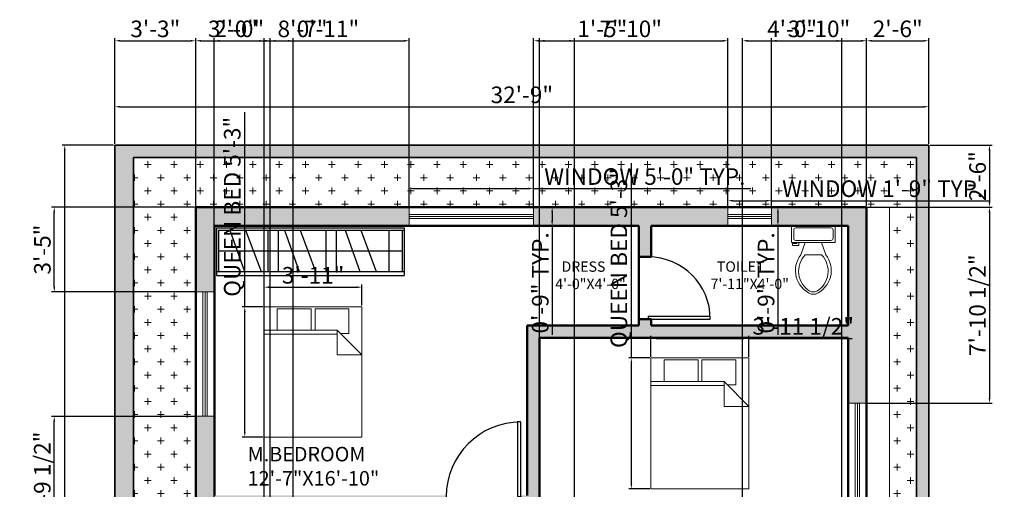
# Model space of a CAD drawing. Units: inches. Extents: x 1369 to 1844, y 2136 to 2743.
# Tile 4 of 4: x 1369 to 1844, y 2517 to 2743. Entities that reach past the tile are written whole.
import ezdxf

# ---------------------------------------------------------------- set-up
doc = ezdxf.new("R2010")
doc.units = ezdxf.units.IN
for name, color, linetype, lineweight in [('A-ANNO-DIMS', 2, 'Continuous', 18), ('A-AREA-IDEN', 7, 'Continuous', 25), ('A-DOOR', 4, 'Continuous', 25), ('A-FLOR-CASE', 8, 'Continuous', 25), ('A-FLOR-FIXT', 9, 'Continuous', 20), ('A-FURN', 8, 'Continuous', 18), ('A-WALL', 7, 'Continuous', 50), ('C-PROP', 7, 'Continuous', 35), ('L-PLNT', 3, 'Continuous', 18)]:
    doc.layers.add(name, color=color, linetype=linetype, lineweight=lineweight)
for name, color, linetype, lineweight, true_color in [('A-GLAZ', 244, 'Continuous', 20, 0x991b1e), ('A-WALL-PATT', 251, 'Continuous', 13, 0x636466), ('C-PROP-PATT', 251, 'Continuous', 13, 0x636466), ('L-PLNT-PATT', 116, 'Continuous', 13, 0x136734)]:
    doc.layers.add(name, color=color, linetype=linetype, lineweight=lineweight, true_color=true_color)
doc.styles.get("Standard").update_dxf_attribs({"font": 'arial.ttf'})
doc.dimstyles.new('ISO-25', dxfattribs={"dimtxt": 8, "dimasz": 2.5, "dimexe": 1.25, "dimexo": 0.625, "dimtad": 1, "dimlunit": 3, "dimtxsty": 'Standard', "dimcen": 2.5, "dimadec": 0, "dimazin": 0, "dimtfac": 1, "dimtmove": 0, "dimatfit": 3, "dimfxl": 1, "dimarcsym": 0})

# ---------------------------------------------------------------- blocks, each defined once
blk = doc.blocks.new('*U2')
for p, q in [((0, 0), (0, -6)), ((-40, 0), (-40, -6))]:
    blk.add_line(p, q)
blk.add_lwpolyline([(0, 0), (0, 40), (-1.75, 40), (-1.75, 0)], close=True)
blk.add_arc((0, 0), 40, 90, 180)
blk = doc.blocks.new('*U4')
for p, q in [((-40, 0), (-40, -6)), ((0, 0), (0, -6))]:
    blk.add_line(p, q)
blk.add_lwpolyline([(0, 0), (0, 40), (-1.75, 40), (-1.75, 0)], close=True)
blk.add_arc((0, 0), 40, 90, 180)
blk = doc.blocks.new('Bed - Queen')
for p, q in [((0, -80.00003), (0, 0)), ((0, 0), (59.99999, 0)), ((59.99999, 0), (59.99999, -80.00003)), ((7.99999, -1.2), (28.79998, -1.2)), ((7.99999, -14.4), (7.99999, -1.2)), ((28.79998, -1.2), (28.79998, -14.4)), ((31.19999, -1.2), (51.99999, -1.2)), ((31.19999, -14.4), (31.19999, -1.2)), ((51.99999, -1.2), (51.99999, -16.4)), ((0, -14.4), (44.8, -14.4)), ((44.8, -16.8), (0, -16.8)), ((59.99999, -29.6), (44.8, -14.4)), ((44.8, -14.4), (44.8, -29.6)), ((51.99999, -16.4), (46.79936, -16.4)), ((44.8, -29.6), (59.99999, -29.6)), ((59.99999, -80.00003), (0, -80.00003))]:
    blk.add_line(p, q)
blk = doc.blocks.new('*U8')
for p, q in [((9.5, -6), (9.5, -2)), ((-10, -8.5), (-8, -8.5)), ((-10, -9.5), (-10, -8.5)), ((-7, -9.5), (-10, -9.5)), ((-8, -8.5), (-8, -8)), ((-7, -8), (-7, -9.5)), ((-4, -8), (-6, -14)), ((4, -8), (6, -14)), ((4, -14), (-4, -14))]:
    blk.add_line(p, q)
blk.add_lwpolyline([(10.5, -8), (10.5, 0), (-10.5, 0), (-10.5, -8)], close=True)
for points in [[(-9.5, -2), (-9.5, -6)], [(8.5, -1), (-8.5, -1)], [(-8.5, -7), (8.5, -7)]]:
    blk.add_lwpolyline(points)
for centre, radius, start, end in [((-8.62, -1.88), 0.884, 81.8699, 188.1301), ((8.62, -1.88), 0.884, 351.8699, 98.1301), ((-8.62, -6.12), 0.884, 171.8699, 278.1301), ((8.62, -6.12), 0.884, 261.8699, 8.1301), ((3.52, -21.58), 12.17, 141.4691, 247.9714), ((4.2, -21.82), 11.33, 136.3677, 238.9468), ((-3.52, -21.58), 12.17, 292.0284, 38.5307), ((-4.2, -21.82), 11.33, 301.053, 43.6321), ((0, -27.88), 4, 245.7318, 294.2682), ((0, -29), 4, 254.8605, 285.1395)]:
    blk.add_arc(centre, radius, start, end)
blk = doc.blocks.new('*D12')
at = {"layer": 'A-ANNO-DIMS', "color": 0, "lineweight": -2, "transparency": 16777216}
for p, q in [((1413.89, 2682.76), (1389.03, 2682.76)), ((1390.28, 2175.26), (1390.28, 2680.26)), ((1413.89, 2172.76), (1389.03, 2172.76))]:
    blk.add_line(p, q, dxfattribs=at)
at = {"layer": 'A-ANNO-DIMS', "color": 0, "transparency": 16777216}
for points in [[(1389.86, 2680.26), (1390.69, 2680.26), (1390.28, 2682.76)], [(1389.86, 2175.26), (1390.69, 2175.26), (1390.28, 2172.76)]]:
    blk.add_solid(points, dxfattribs=at)
at = {"layer": 'Defpoints', "color": 0, "transparency": 16777216}
for p in [(1390.28, 2682.76), (1414.51, 2682.76), (1414.51, 2172.76)]:
    blk.add_point(p, dxfattribs=at)
at = {"layer": 'A-ANNO-DIMS', "color": 0, "transparency": 16777216, "insert": (1385.57, 2427.76), "char_height": 8, "attachment_point": 5, "rotation": 90}
blk.add_mtext('42\'-6"', dxfattribs=at)
blk = doc.blocks.new('*D13')
at = {"layer": 'A-ANNO-DIMS', "color": 0, "lineweight": -2, "transparency": 16777216}
for p, q in [((1414.51, 2683.38), (1414.51, 2702.48)), ((1417.01, 2701.23), (1805.01, 2701.23)), ((1807.51, 2683.38), (1807.51, 2702.48))]:
    blk.add_line(p, q, dxfattribs=at)
at = {"layer": 'A-ANNO-DIMS', "color": 0, "transparency": 16777216}
for points in [[(1417.01, 2701.65), (1417.01, 2700.81), (1414.51, 2701.23)], [(1805.01, 2701.65), (1805.01, 2700.81), (1807.51, 2701.23)]]:
    blk.add_solid(points, dxfattribs=at)
at = {"layer": 'Defpoints', "color": 0, "transparency": 16777216}
for p in [(1807.51, 2701.23), (1414.51, 2682.76), (1807.51, 2682.76)]:
    blk.add_point(p, dxfattribs=at)
at = {"layer": 'A-ANNO-DIMS', "color": 0, "transparency": 16777216, "insert": (1611.01, 2705.94), "char_height": 8, "attachment_point": 5}
blk.add_mtext('32\'-9"', dxfattribs=at)
blk = doc.blocks.new('WIN-60IN')
for p, q in [((3.5, 0), (3.5, 60)), ((4.5, 0), (4.5, 60)), ((5.5, 0), (5.5, 60))]:
    blk.add_line(p, q)
blk.add_lwpolyline([(0, 60), (9, 60), (9, 0), (0, 0)], close=True)
blk = doc.blocks.new('WIN-21IN')
for p, q in [((3.5, 21), (3.5, 0)), ((4.5, 21), (4.5, 0)), ((5.5, 21), (5.5, 0))]:
    blk.add_line(p, q)
blk.add_lwpolyline([(0, 21), (9, 21), (9, 0), (0, 0)], close=True)
blk = doc.blocks.new('*D16')
at = {"layer": 'A-ANNO-DIMS', "color": 0, "lineweight": -2, "transparency": 16777216}
for p, q in [((1556.64, 2653.38), (1556.64, 2663.01)), ((1616.64, 2653.38), (1616.64, 2663.01)), ((1559.14, 2661.76), (1614.14, 2661.76)), ((1616.64, 2661.76), (1721.63, 2661.76))]:
    blk.add_line(p, q, dxfattribs=at)
at = {"layer": 'A-ANNO-DIMS', "color": 0, "transparency": 16777216}
for points in [[(1559.14, 2662.17), (1559.14, 2661.34), (1556.64, 2661.76)], [(1614.14, 2662.17), (1614.14, 2661.34), (1616.64, 2661.76)]]:
    blk.add_solid(points, dxfattribs=at)
at = {"layer": 'Defpoints', "color": 0, "transparency": 16777216}
for p in [(1616.64, 2661.76), (1556.64, 2652.76), (1616.64, 2652.76)]:
    blk.add_point(p, dxfattribs=at)
at = {"layer": 'A-ANNO-DIMS', "color": 0, "transparency": 16777216, "insert": (1670.38, 2666.52), "char_height": 8, "attachment_point": 5}
blk.add_mtext('WINDOW 5\'-0" TYP.', dxfattribs=at)
blk = doc.blocks.new('*D17')
at = {"layer": 'A-ANNO-DIMS', "color": 0, "lineweight": -2, "transparency": 16777216}
for p, q in [((1617.27, 2652.76), (1626.89, 2652.76)), ((1625.64, 2650.26), (1625.64, 2646.26)), ((1617.27, 2643.76), (1626.89, 2643.76)), ((1625.64, 2643.76), (1625.64, 2591.24))]:
    blk.add_line(p, q, dxfattribs=at)
at = {"layer": 'A-ANNO-DIMS', "color": 0, "transparency": 16777216}
for points in [[(1625.23, 2650.26), (1626.06, 2650.26), (1625.64, 2652.76)], [(1625.23, 2646.26), (1626.06, 2646.26), (1625.64, 2643.76)]]:
    blk.add_solid(points, dxfattribs=at)
at = {"layer": 'Defpoints', "color": 0, "transparency": 16777216}
for p in [(1616.64, 2652.76), (1616.64, 2643.76), (1625.64, 2643.76)]:
    blk.add_point(p, dxfattribs=at)
at = {"layer": 'A-ANNO-DIMS', "color": 0, "transparency": 16777216, "insert": (1620.93, 2616.25), "char_height": 8, "attachment_point": 5, "rotation": 90}
blk.add_mtext('0\'-9" TYP.', dxfattribs=at)
blk = doc.blocks.new('*D18')
at = {"layer": 'A-ANNO-DIMS', "color": 0, "lineweight": -2, "transparency": 16777216}
for p, q in [((1710.51, 2653.38), (1710.51, 2657.16)), ((1713.01, 2655.91), (1729.01, 2655.91)), ((1731.51, 2653.38), (1731.51, 2657.16)), ((1731.51, 2655.91), (1836.49, 2655.91))]:
    blk.add_line(p, q, dxfattribs=at)
at = {"layer": 'A-ANNO-DIMS', "color": 0, "transparency": 16777216}
for points in [[(1713.01, 2656.32), (1713.01, 2655.49), (1710.51, 2655.91)], [(1729.01, 2656.32), (1729.01, 2655.49), (1731.51, 2655.91)]]:
    blk.add_solid(points, dxfattribs=at)
at = {"layer": 'Defpoints', "color": 0, "transparency": 16777216}
for p in [(1731.51, 2655.91), (1710.51, 2652.76), (1731.51, 2652.76)]:
    blk.add_point(p, dxfattribs=at)
at = {"layer": 'A-ANNO-DIMS', "color": 0, "transparency": 16777216, "insert": (1785.25, 2660.67), "char_height": 8, "attachment_point": 5}
blk.add_mtext('WINDOW 1\'-9" TYP.', dxfattribs=at)
blk = doc.blocks.new('*D19')
at = {"layer": 'A-ANNO-DIMS', "color": 0, "lineweight": -2, "transparency": 16777216}
for p, q in [((1732.14, 2652.76), (1735.91, 2652.76)), ((1734.66, 2650.26), (1734.66, 2646.26)), ((1732.14, 2643.76), (1735.91, 2643.76)), ((1734.66, 2643.76), (1734.66, 2591.24))]:
    blk.add_line(p, q, dxfattribs=at)
at = {"layer": 'A-ANNO-DIMS', "color": 0, "transparency": 16777216}
for points in [[(1734.24, 2650.26), (1735.08, 2650.26), (1734.66, 2652.76)], [(1734.24, 2646.26), (1735.08, 2646.26), (1734.66, 2643.76)]]:
    blk.add_solid(points, dxfattribs=at)
at = {"layer": 'Defpoints', "color": 0, "transparency": 16777216}
for p in [(1731.51, 2652.76), (1731.51, 2643.76), (1734.66, 2643.76)]:
    blk.add_point(p, dxfattribs=at)
at = {"layer": 'A-ANNO-DIMS', "color": 0, "transparency": 16777216, "insert": (1729.95, 2616.25), "char_height": 8, "attachment_point": 5, "rotation": 90}
blk.add_mtext('0\'-9" TYP.', dxfattribs=at)
blk = doc.blocks.new('*D20')
at = {"layer": 'A-ANNO-DIMS', "color": 0, "lineweight": -2, "transparency": 16777216}
for p, q in [((1663.89, 2580.04), (1663.89, 2673.97)), ((1672.74, 2580.04), (1662.64, 2580.04)), ((1663.89, 2519.43), (1663.89, 2577.54)), ((1672.74, 2516.93), (1662.64, 2516.93))]:
    blk.add_line(p, q, dxfattribs=at)
at = {"layer": 'A-ANNO-DIMS', "color": 0, "transparency": 16777216}
for points in [[(1663.48, 2577.54), (1664.31, 2577.54), (1663.89, 2580.04)], [(1663.48, 2519.43), (1664.31, 2519.43), (1663.89, 2516.93)]]:
    blk.add_solid(points, dxfattribs=at)
at = {"layer": 'Defpoints', "color": 0, "transparency": 16777216}
for p in [(1663.89, 2580.04), (1673.36, 2580.04), (1673.36, 2516.93)]:
    blk.add_point(p, dxfattribs=at)
at = {"layer": 'A-ANNO-DIMS', "color": 0, "transparency": 16777216, "insert": (1658.89, 2628.25), "char_height": 8, "attachment_point": 5, "rotation": 90}
blk.add_mtext('QUEEN BED 5\'-3"', dxfattribs=at)
blk = doc.blocks.new('*D21')
at = {"layer": 'A-ANNO-DIMS', "color": 0, "lineweight": -2, "transparency": 16777216}
for p, q in [((1673.36, 2580.66), (1673.36, 2590.75)), ((1675.86, 2589.5), (1718.19, 2589.5)), ((1720.69, 2580.66), (1720.69, 2590.75)), ((1720.69, 2589.5), (1770.56, 2589.5))]:
    blk.add_line(p, q, dxfattribs=at)
at = {"layer": 'A-ANNO-DIMS', "color": 0, "transparency": 16777216}
for points in [[(1675.86, 2589.92), (1675.86, 2589.09), (1673.36, 2589.5)], [(1718.19, 2589.92), (1718.19, 2589.09), (1720.69, 2589.5)]]:
    blk.add_solid(points, dxfattribs=at)
at = {"layer": 'Defpoints', "color": 0, "transparency": 16777216}
for p in [(1720.69, 2589.5), (1673.36, 2580.04), (1720.69, 2580.04)]:
    blk.add_point(p, dxfattribs=at)
at = {"layer": 'A-ANNO-DIMS', "color": 0, "transparency": 16777216, "insert": (1746.87, 2594.27), "char_height": 8, "attachment_point": 5}
blk.add_mtext('3\'-11 1/2"', dxfattribs=at)
blk = doc.blocks.new('*D22')
at = {"layer": 'A-ANNO-DIMS', "color": 0, "lineweight": -2, "transparency": 16777216}
for p, q in [((1477.21, 2604.75), (1477.21, 2698.68)), ((1486.01, 2604.75), (1475.96, 2604.75)), ((1477.21, 2544.39), (1477.21, 2602.25)), ((1486.01, 2541.89), (1475.96, 2541.89))]:
    blk.add_line(p, q, dxfattribs=at)
at = {"layer": 'A-ANNO-DIMS', "color": 0, "transparency": 16777216}
for points in [[(1476.79, 2602.25), (1477.63, 2602.25), (1477.21, 2604.75)], [(1476.79, 2544.39), (1477.63, 2544.39), (1477.21, 2541.89)]]:
    blk.add_solid(points, dxfattribs=at)
at = {"layer": 'Defpoints', "color": 0, "transparency": 16777216}
for p in [(1477.21, 2604.75), (1486.64, 2604.75), (1486.64, 2541.89)]:
    blk.add_point(p, dxfattribs=at)
at = {"layer": 'A-ANNO-DIMS', "color": 0, "transparency": 16777216, "insert": (1472.2, 2652.97), "char_height": 8, "attachment_point": 5, "rotation": 90}
blk.add_mtext('QUEEN BED 5\'-3"', dxfattribs=at)
blk = doc.blocks.new('*D23')
at = {"layer": 'A-ANNO-DIMS', "color": 0, "lineweight": -2, "transparency": 16777216}
for p, q in [((1486.64, 2605.38), (1486.64, 2615.43)), ((1533.78, 2605.38), (1533.78, 2615.43)), ((1489.14, 2614.18), (1531.28, 2614.18))]:
    blk.add_line(p, q, dxfattribs=at)
at = {"layer": 'A-ANNO-DIMS', "color": 0, "transparency": 16777216}
for points in [[(1489.14, 2614.6), (1489.14, 2613.76), (1486.64, 2614.18)], [(1531.28, 2614.6), (1531.28, 2613.76), (1533.78, 2614.18)]]:
    blk.add_solid(points, dxfattribs=at)
at = {"layer": 'Defpoints', "color": 0, "transparency": 16777216}
for p in [(1533.78, 2614.18), (1486.64, 2604.75), (1533.78, 2604.75)]:
    blk.add_point(p, dxfattribs=at)
at = {"layer": 'A-ANNO-DIMS', "color": 0, "transparency": 16777216, "insert": (1510.21, 2618.89), "char_height": 8, "attachment_point": 5}
blk.add_mtext('3\'-11"', dxfattribs=at)
blk = doc.blocks.new('*D26')
at = {"layer": 'A-ANNO-DIMS', "color": 0, "lineweight": -2, "transparency": 16777216}
for p, q in [((1414.51, 2683.38), (1414.51, 2734.31)), ((1453.51, 2653.38), (1453.51, 2734.31)), ((1417.01, 2733.06), (1451.01, 2733.06))]:
    blk.add_line(p, q, dxfattribs=at)
at = {"layer": 'A-ANNO-DIMS', "color": 0, "transparency": 16777216}
for points in [[(1417.01, 2733.47), (1417.01, 2732.64), (1414.51, 2733.06)], [(1451.01, 2733.47), (1451.01, 2732.64), (1453.51, 2733.06)]]:
    blk.add_solid(points, dxfattribs=at)
at = {"layer": 'Defpoints', "color": 0, "transparency": 16777216}
for p in [(1453.51, 2733.06), (1414.51, 2682.76), (1453.51, 2652.76)]:
    blk.add_point(p, dxfattribs=at)
at = {"layer": 'A-ANNO-DIMS', "color": 0, "transparency": 16777216, "insert": (1434.01, 2737.77), "char_height": 8, "attachment_point": 5}
blk.add_mtext('3\'-3"', dxfattribs=at)
blk = doc.blocks.new('*D27')
at = {"layer": 'A-ANNO-DIMS', "color": 0, "lineweight": -2, "transparency": 16777216}
for p, q in [((1453.51, 2653.38), (1453.51, 2734.31)), ((1556.64, 2653.38), (1556.64, 2734.31)), ((1456.01, 2733.06), (1554.14, 2733.06))]:
    blk.add_line(p, q, dxfattribs=at)
at = {"layer": 'A-ANNO-DIMS', "color": 0, "transparency": 16777216}
for points in [[(1456.01, 2733.47), (1456.01, 2732.64), (1453.51, 2733.06)], [(1554.14, 2733.47), (1554.14, 2732.64), (1556.64, 2733.06)]]:
    blk.add_solid(points, dxfattribs=at)
at = {"layer": 'Defpoints', "color": 0, "transparency": 16777216}
for p in [(1556.64, 2733.06), (1453.51, 2652.76), (1556.64, 2652.76)]:
    blk.add_point(p, dxfattribs=at)
at = {"layer": 'A-ANNO-DIMS', "color": 0, "transparency": 16777216, "insert": (1505.08, 2737.77), "char_height": 8, "attachment_point": 5}
blk.add_mtext('8\'-7"', dxfattribs=at)
blk = doc.blocks.new('*D28')
at = {"layer": 'A-ANNO-DIMS', "color": 0, "lineweight": -2, "transparency": 16777216}
for p, q in [((1616.64, 2653.38), (1616.64, 2734.31)), ((1710.51, 2653.38), (1710.51, 2734.31)), ((1619.14, 2733.06), (1708.01, 2733.06))]:
    blk.add_line(p, q, dxfattribs=at)
at = {"layer": 'A-ANNO-DIMS', "color": 0, "transparency": 16777216}
for points in [[(1619.14, 2733.47), (1619.14, 2732.64), (1616.64, 2733.06)], [(1708.01, 2733.47), (1708.01, 2732.64), (1710.51, 2733.06)]]:
    blk.add_solid(points, dxfattribs=at)
at = {"layer": 'Defpoints', "color": 0, "transparency": 16777216}
for p in [(1710.51, 2733.06), (1616.64, 2652.76), (1710.51, 2652.76)]:
    blk.add_point(p, dxfattribs=at)
at = {"layer": 'A-ANNO-DIMS', "color": 0, "transparency": 16777216, "insert": (1663.58, 2737.77), "char_height": 8, "attachment_point": 5}
blk.add_mtext('7\'-10"', dxfattribs=at)
blk = doc.blocks.new('*D29')
at = {"layer": 'A-ANNO-DIMS', "color": 0, "lineweight": -2, "transparency": 16777216}
for p, q in [((1731.51, 2653.38), (1731.51, 2734.31)), ((1777.51, 2653.38), (1777.51, 2734.31)), ((1734.01, 2733.06), (1775.01, 2733.06))]:
    blk.add_line(p, q, dxfattribs=at)
at = {"layer": 'A-ANNO-DIMS', "color": 0, "transparency": 16777216}
for points in [[(1734.01, 2733.47), (1734.01, 2732.64), (1731.51, 2733.06)], [(1775.01, 2733.47), (1775.01, 2732.64), (1777.51, 2733.06)]]:
    blk.add_solid(points, dxfattribs=at)
at = {"layer": 'Defpoints', "color": 0, "transparency": 16777216}
for p in [(1777.51, 2733.06), (1731.51, 2652.76), (1777.51, 2652.76)]:
    blk.add_point(p, dxfattribs=at)
at = {"layer": 'A-ANNO-DIMS', "color": 0, "transparency": 16777216, "insert": (1754.51, 2737.77), "char_height": 8, "attachment_point": 5}
blk.add_mtext('3\'-10"', dxfattribs=at)
blk = doc.blocks.new('*D30')
at = {"layer": 'A-ANNO-DIMS', "color": 0, "lineweight": -2, "transparency": 16777216}
for p, q in [((1777.51, 2653.38), (1777.51, 2734.31)), ((1807.51, 2683.38), (1807.51, 2734.31)), ((1780.01, 2733.06), (1805.01, 2733.06))]:
    blk.add_line(p, q, dxfattribs=at)
at = {"layer": 'A-ANNO-DIMS', "color": 0, "transparency": 16777216}
for points in [[(1780.01, 2733.47), (1780.01, 2732.64), (1777.51, 2733.06)], [(1805.01, 2733.47), (1805.01, 2732.64), (1807.51, 2733.06)]]:
    blk.add_solid(points, dxfattribs=at)
at = {"layer": 'Defpoints', "color": 0, "transparency": 16777216}
for p in [(1807.51, 2733.06), (1807.51, 2682.76), (1777.51, 2652.76)]:
    blk.add_point(p, dxfattribs=at)
at = {"layer": 'A-ANNO-DIMS', "color": 0, "transparency": 16777216, "insert": (1792.51, 2737.77), "char_height": 8, "attachment_point": 5}
blk.add_mtext('2\'-6"', dxfattribs=at)
blk = doc.blocks.new('*D31')
at = {"layer": 'A-ANNO-DIMS', "color": 0, "lineweight": -2, "transparency": 16777216}
for p, q in [((1808.14, 2682.76), (1838.06, 2682.76)), ((1836.81, 2680.26), (1836.81, 2655.26)), ((1778.14, 2652.76), (1838.06, 2652.76))]:
    blk.add_line(p, q, dxfattribs=at)
at = {"layer": 'A-ANNO-DIMS', "color": 0, "transparency": 16777216}
for points in [[(1836.39, 2680.26), (1837.23, 2680.26), (1836.81, 2682.76)], [(1836.39, 2655.26), (1837.23, 2655.26), (1836.81, 2652.76)]]:
    blk.add_solid(points, dxfattribs=at)
at = {"layer": 'Defpoints', "color": 0, "transparency": 16777216}
for p in [(1807.51, 2682.76), (1777.51, 2652.76), (1836.81, 2652.76)]:
    blk.add_point(p, dxfattribs=at)
at = {"layer": 'A-ANNO-DIMS', "color": 0, "transparency": 16777216, "insert": (1832.1, 2667.76), "char_height": 8, "attachment_point": 5, "rotation": 90}
blk.add_mtext('2\'-6"', dxfattribs=at)
blk = doc.blocks.new('*D32')
at = {"layer": 'A-ANNO-DIMS', "color": 0, "lineweight": -2, "transparency": 16777216}
for p, q in [((1778.14, 2652.76), (1838.06, 2652.76)), ((1836.81, 2650.26), (1836.81, 2560.76)), ((1778.14, 2558.26), (1838.06, 2558.26))]:
    blk.add_line(p, q, dxfattribs=at)
at = {"layer": 'A-ANNO-DIMS', "color": 0, "transparency": 16777216}
for points in [[(1836.39, 2650.26), (1837.23, 2650.26), (1836.81, 2652.76)], [(1836.39, 2560.76), (1837.23, 2560.76), (1836.81, 2558.26)]]:
    blk.add_solid(points, dxfattribs=at)
at = {"layer": 'Defpoints', "color": 0, "transparency": 16777216}
for p in [(1777.51, 2652.76), (1777.51, 2558.26), (1836.81, 2558.26)]:
    blk.add_point(p, dxfattribs=at)
at = {"layer": 'A-ANNO-DIMS', "color": 0, "transparency": 16777216, "insert": (1832.05, 2605.51), "char_height": 8, "attachment_point": 5, "rotation": 90}
blk.add_mtext('7\'-10 1/2"', dxfattribs=at)
blk = doc.blocks.new('*D40')
at = {"layer": 'A-ANNO-DIMS', "color": 0, "lineweight": -2, "transparency": 16777216}
for p, q in [((1452.89, 2551.88), (1383.96, 2551.88)), ((1385.21, 2496.76), (1385.21, 2549.38)), ((1452.89, 2494.26), (1383.96, 2494.26))]:
    blk.add_line(p, q, dxfattribs=at)
at = {"layer": 'A-ANNO-DIMS', "color": 0, "transparency": 16777216}
for points in [[(1384.79, 2549.38), (1385.63, 2549.38), (1385.21, 2551.88)], [(1384.79, 2496.76), (1385.63, 2496.76), (1385.21, 2494.26)]]:
    blk.add_solid(points, dxfattribs=at)
at = {"layer": 'Defpoints', "color": 0, "transparency": 16777216}
for p in [(1385.21, 2551.88), (1453.51, 2551.88), (1453.51, 2494.26)]:
    blk.add_point(p, dxfattribs=at)
at = {"layer": 'A-ANNO-DIMS', "color": 0, "transparency": 16777216, "insert": (1380.45, 2523.07), "char_height": 8, "attachment_point": 5, "rotation": 90}
blk.add_mtext('4\'-9 1/2"', dxfattribs=at)
blk = doc.blocks.new('*D41')
at = {"layer": 'A-ANNO-DIMS', "color": 0, "lineweight": -2, "transparency": 16777216}
for p, q in [((1452.89, 2652.76), (1383.96, 2652.76)), ((1385.21, 2614.38), (1385.21, 2650.26)), ((1452.89, 2611.88), (1383.96, 2611.88))]:
    blk.add_line(p, q, dxfattribs=at)
at = {"layer": 'A-ANNO-DIMS', "color": 0, "transparency": 16777216}
for points in [[(1384.79, 2650.26), (1385.63, 2650.26), (1385.21, 2652.76)], [(1384.79, 2614.38), (1385.63, 2614.38), (1385.21, 2611.88)]]:
    blk.add_solid(points, dxfattribs=at)
at = {"layer": 'Defpoints', "color": 0, "transparency": 16777216}
for p in [(1385.21, 2652.76), (1453.51, 2652.76), (1453.51, 2611.88)]:
    blk.add_point(p, dxfattribs=at)
at = {"layer": 'A-ANNO-DIMS', "color": 0, "transparency": 16777216, "insert": (1380.5, 2632.32), "char_height": 8, "attachment_point": 5, "rotation": 90}
blk.add_mtext('3\'-5"', dxfattribs=at)
blk = doc.blocks.new('*D45')
at = {"layer": 'A-ANNO-DIMS', "color": 0, "lineweight": -2, "transparency": 16777216}
for p, q in [((1619.51, 2326.38), (1619.51, 2734.31)), ((1636.5, 2326.38), (1636.5, 2734.31)), ((1622.01, 2733.06), (1634, 2733.06)), ((1636.5, 2733.06), (1660.77, 2733.06))]:
    blk.add_line(p, q, dxfattribs=at)
at = {"layer": 'A-ANNO-DIMS', "color": 0, "transparency": 16777216}
for points in [[(1622.01, 2733.47), (1622.01, 2732.64), (1619.51, 2733.06)], [(1634, 2733.47), (1634, 2732.64), (1636.5, 2733.06)]]:
    blk.add_solid(points, dxfattribs=at)
at = {"layer": 'Defpoints', "color": 0, "transparency": 16777216}
for p in [(1636.5, 2733.06), (1619.51, 2325.76), (1636.5, 2325.76)]:
    blk.add_point(p, dxfattribs=at)
at = {"layer": 'A-ANNO-DIMS', "color": 0, "transparency": 16777216, "insert": (1649.88, 2737.77), "char_height": 8, "attachment_point": 5}
blk.add_mtext('1\'-5"', dxfattribs=at)
blk = doc.blocks.new('*D46')
at = {"layer": 'A-ANNO-DIMS', "color": 0, "lineweight": -2, "transparency": 16777216}
for p, q in [((1717.51, 2326.38), (1717.51, 2734.31)), ((1765.51, 2326.38), (1765.51, 2734.31)), ((1720.01, 2733.06), (1763.01, 2733.06))]:
    blk.add_line(p, q, dxfattribs=at)
at = {"layer": 'A-ANNO-DIMS', "color": 0, "transparency": 16777216}
for points in [[(1720.01, 2733.47), (1720.01, 2732.64), (1717.51, 2733.06)], [(1763.01, 2733.47), (1763.01, 2732.64), (1765.51, 2733.06)]]:
    blk.add_solid(points, dxfattribs=at)
at = {"layer": 'Defpoints', "color": 0, "transparency": 16777216}
for p in [(1765.51, 2733.06), (1717.51, 2325.76), (1765.51, 2325.76)]:
    blk.add_point(p, dxfattribs=at)
at = {"layer": 'A-ANNO-DIMS', "color": 0, "transparency": 16777216, "insert": (1741.51, 2737.77), "char_height": 8, "attachment_point": 5}
blk.add_mtext('4\'-0"', dxfattribs=at)
blk = doc.blocks.new('*D54')
at = {"layer": 'A-ANNO-DIMS', "color": 0, "lineweight": -2, "transparency": 16777216}
for p, q in [((1462.51, 2268.38), (1462.51, 2734.31)), ((1486.51, 2292.38), (1486.51, 2734.31)), ((1465.01, 2733.06), (1484.01, 2733.06))]:
    blk.add_line(p, q, dxfattribs=at)
at = {"layer": 'A-ANNO-DIMS', "color": 0, "transparency": 16777216}
for points in [[(1465.01, 2733.47), (1465.01, 2732.64), (1462.51, 2733.06)], [(1484.01, 2733.47), (1484.01, 2732.64), (1486.51, 2733.06)]]:
    blk.add_solid(points, dxfattribs=at)
at = {"layer": 'Defpoints', "color": 0, "transparency": 16777216}
for p in [(1486.51, 2733.06), (1486.51, 2291.76), (1462.51, 2267.76)]:
    blk.add_point(p, dxfattribs=at)
at = {"layer": 'A-ANNO-DIMS', "color": 0, "transparency": 16777216, "insert": (1474.51, 2737.77), "char_height": 8, "attachment_point": 5}
blk.add_mtext('2\'-0"', dxfattribs=at)
blk = doc.blocks.new('*D55')
at = {"layer": 'A-ANNO-DIMS', "color": 0, "lineweight": -2, "transparency": 16777216}
for p, q in [((1453.51, 2179.38), (1453.51, 2734.31)), ((1489.51, 2179.38), (1489.51, 2734.31)), ((1456.01, 2733.06), (1487.01, 2733.06))]:
    blk.add_line(p, q, dxfattribs=at)
at = {"layer": 'A-ANNO-DIMS', "color": 0, "transparency": 16777216}
for points in [[(1456.01, 2733.47), (1456.01, 2732.64), (1453.51, 2733.06)], [(1487.01, 2733.47), (1487.01, 2732.64), (1489.51, 2733.06)]]:
    blk.add_solid(points, dxfattribs=at)
at = {"layer": 'Defpoints', "color": 0, "transparency": 16777216}
for p in [(1489.51, 2733.06), (1453.51, 2178.76), (1489.51, 2178.76)]:
    blk.add_point(p, dxfattribs=at)
at = {"layer": 'A-ANNO-DIMS', "color": 0, "transparency": 16777216, "insert": (1471.51, 2737.77), "char_height": 8, "attachment_point": 5}
blk.add_mtext('3\'-0"', dxfattribs=at)
blk = doc.blocks.new('*D56')
at = {"layer": 'A-ANNO-DIMS', "color": 0, "lineweight": -2, "transparency": 16777216}
for p, q in [((1489.51, 2222.38), (1489.51, 2734.31)), ((1500.51, 2222.38), (1500.51, 2734.31)), ((1492.01, 2733.06), (1498.01, 2733.06)), ((1500.51, 2733.06), (1531.74, 2733.06))]:
    blk.add_line(p, q, dxfattribs=at)
at = {"layer": 'A-ANNO-DIMS', "color": 0, "transparency": 16777216}
for points in [[(1492.01, 2733.47), (1492.01, 2732.64), (1489.51, 2733.06)], [(1498.01, 2733.47), (1498.01, 2732.64), (1500.51, 2733.06)]]:
    blk.add_solid(points, dxfattribs=at)
at = {"layer": 'Defpoints', "color": 0, "transparency": 16777216}
for p in [(1500.51, 2733.06), (1489.51, 2221.76), (1500.51, 2221.76)]:
    blk.add_point(p, dxfattribs=at)
at = {"layer": 'A-ANNO-DIMS', "color": 0, "transparency": 16777216, "insert": (1517.38, 2737.77), "char_height": 8, "attachment_point": 5}
blk.add_mtext('0\'-11"', dxfattribs=at)

msp = doc.modelspace()

# ---------------------------------------------------------------- hatches: boundary and pattern name
at = {"layer": 'A-WALL-PATT'}
h = msp.add_hatch(color=256, dxfattribs=at)
h.dxf.hatch_style = 1
h.paths.add_polyline_path([(1619.511, 2460.756), (1768.511, 2460.756), (1768.511, 2444.065), (1777.511, 2444.065), (1777.511, 2498.256), (1768.511, 2498.256), (1768.511, 2466.756), (1619.511, 2466.756), (1619.511, 2469.756), (1614.511, 2469.756), (1613.511, 2469.756), (1613.511, 2433.756), (1619.511, 2433.756)])
h.paths.add_polyline_path([(1480.511, 2453.756), (1560.511, 2453.756), (1560.511, 2474.756), (1556.011, 2474.756), (1554.511, 2474.756), (1554.511, 2459.756), (1462.511, 2459.756), (1462.511, 2473.256), (1453.511, 2473.256), (1453.511, 2453.756), (1471.511, 2453.756), (1471.511, 2390.756), (1480.511, 2390.756)])
h.paths.add_polyline_path([(1574.511, 2513.156), (1574.511, 2513.756), (1462.511, 2513.756), (1462.511, 2551.882), (1453.511, 2551.882), (1453.511, 2494.256), (1462.511, 2494.256), (1462.511, 2507.756), (1554.511, 2507.756), (1554.511, 2504.756), (1556.011, 2504.756), (1560.511, 2504.756), (1560.511, 2507.756), (1574.511, 2507.756)])
h.paths.add_polyline_path([(1462.511, 2351.756), (1480.511, 2351.756), (1480.511, 2357.756), (1480.511, 2360.756), (1476.011, 2360.756), (1471.511, 2360.756), (1471.511, 2357.756), (1453.511, 2357.756), (1453.511, 2258.756), (1508.011, 2258.756), (1508.011, 2267.756), (1462.511, 2267.756)])
h.paths.add_polyline_path([(1619.511, 2357.756), (1592.511, 2357.756), (1592.511, 2351.756), (1613.511, 2351.756), (1613.511, 2267.756), (1568.011, 2267.756), (1568.011, 2258.756), (1619.511, 2258.756), (1619.511, 2316.756), (1636.503, 2316.756), (1636.503, 2325.756), (1619.511, 2325.756)])
h.paths.add_polyline_path([(1717.511, 2323.956), (1717.511, 2325.756), (1696.503, 2325.756), (1696.503, 2316.756), (1717.511, 2316.756)])
h.paths.add_polyline_path([(1777.511, 2384.065), (1768.511, 2384.065), (1768.511, 2325.756), (1765.511, 2325.756), (1765.511, 2323.956), (1765.511, 2316.756), (1777.511, 2316.756)])
h.paths.add_polyline_path([(1777.511, 2652.756), (1731.511, 2652.756), (1731.511, 2643.756), (1768.511, 2643.756), (1768.511, 2595.756), (1673.511, 2595.756), (1673.511, 2598.756), (1672.011, 2598.756), (1667.511, 2598.756), (1667.511, 2595.756), (1613.511, 2595.756), (1613.511, 2513.756), (1610.511, 2513.756), (1610.511, 2513.156), (1610.511, 2507.756), (1613.511, 2507.756), (1613.511, 2505.756), (1619.511, 2505.756), (1619.511, 2589.756), (1768.511, 2589.756), (1768.511, 2558.256), (1777.511, 2558.256)])
h.paths.add_polyline_path([(1710.511, 2652.756), (1616.643, 2652.756), (1616.643, 2643.756), (1667.511, 2643.756), (1667.511, 2628.756), (1672.011, 2628.756), (1673.511, 2628.756), (1673.511, 2643.756), (1710.511, 2643.756)], flags=17)
h.paths.add_polyline_path([(1556.643, 2652.756), (1453.511, 2652.756), (1453.511, 2611.882), (1462.511, 2611.882), (1462.511, 2643.756), (1556.643, 2643.756)])
at = {"layer": 'C-PROP-PATT'}
h = msp.add_hatch(color=256, dxfattribs=at)
h.dxf.hatch_style = 1
h.paths.add_polyline_path([(1423.511, 2676.756), (1801.511, 2676.756), (1801.511, 2178.756), (1777.511, 2178.756), (1777.511, 2172.756), (1807.511, 2172.756), (1807.511, 2682.756), (1414.511, 2682.756), (1414.511, 2172.756), (1642.884, 2172.756), (1642.884, 2178.756), (1423.511, 2178.756)])
at = {"layer": 'L-PLNT-PATT'}
h = msp.add_hatch(dxfattribs=at)
h.set_pattern_fill('CROSS', color=256)
h.paths.add_polyline_path([(1453.511, 2652.756), (1777.511, 2652.756), (1788.511, 2652.756), (1788.511, 2178.756), (1801.511, 2178.756), (1801.511, 2676.756), (1423.511, 2676.756), (1423.511, 2453.756), (1453.511, 2453.756)])
h.paths.add_polyline_path([(1453.511, 2350.279), (1423.511, 2350.279), (1423.511, 2178.756), (1453.511, 2178.756), (1453.511, 2258.756)], flags=17)

# ---------------------------------------------------------------- linework, layer by layer
at = {"layer": 'A-FLOR-CASE'}
for p, q in [((1463.511, 2642.756), (1554.241, 2642.756)), ((1463.511, 2642.756), (1463.511, 2619.756)), ((1464.511, 2641.756), (1464.511, 2621.756)), ((1464.511, 2641.756), (1554.241, 2641.756)), ((1469.996, 2641.756), (1477.103, 2621.756)), ((1477.633, 2641.756), (1485.051, 2621.756)), ((1488.366, 2641.756), (1488.366, 2621.756)), ((1493.399, 2641.756), (1493.399, 2621.756)), ((1496.357, 2641.756), (1503.464, 2621.756)), ((1503.994, 2641.756), (1511.412, 2621.756)), ((1516.367, 2641.756), (1516.367, 2621.756)), ((1521.4, 2641.756), (1521.4, 2621.756)), ((1525.657, 2641.756), (1532.764, 2621.756)), ((1533.294, 2641.756), (1540.712, 2621.756)), ((1546.834, 2641.756), (1546.834, 2621.756)), ((1553.241, 2641.756), (1553.241, 2621.756)), ((1554.241, 2642.756), (1554.241, 2619.756)), ((1464.511, 2631.756), (1553.241, 2631.756)), ((1463.511, 2621.756), (1554.241, 2621.756)), ((1463.511, 2619.756), (1554.241, 2619.756))]:
    msp.add_line(p, q, dxfattribs=at)
at = {"layer": 'A-WALL'}
for p, q in [((1453.511, 2652.756), (1453.511, 2453.756)), ((1453.511, 2652.756), (1777.511, 2652.756)), ((1777.511, 2652.756), (1777.511, 2316.756)), ((1462.511, 2643.756), (1462.511, 2513.756)), ((1462.511, 2643.756), (1613.511, 2643.756)), ((1613.511, 2643.756), (1667.511, 2643.756)), ((1667.511, 2643.756), (1667.511, 2595.756)), ((1673.511, 2643.756), (1673.511, 2628.756)), ((1673.511, 2643.756), (1768.511, 2643.756)), ((1768.511, 2643.756), (1768.511, 2595.756)), ((1667.511, 2628.756), (1673.511, 2628.756)), ((1667.511, 2598.756), (1673.511, 2598.756)), ((1673.511, 2598.756), (1673.511, 2595.756)), ((1613.511, 2595.756), (1613.511, 2513.756)), ((1613.511, 2595.756), (1667.511, 2595.756)), ((1673.511, 2595.756), (1768.511, 2595.756)), ((1619.511, 2589.756), (1619.511, 2505.756)), ((1619.511, 2589.756), (1768.511, 2589.756)), ((1768.511, 2589.756), (1768.511, 2466.756))]:
    msp.add_line(p, q, dxfattribs=at)
at = {"layer": 'C-PROP'}
for p, q in [((1414.511, 2682.756), (1414.511, 2172.756)), ((1414.511, 2682.756), (1807.511, 2682.756)), ((1807.511, 2682.756), (1807.511, 2172.756)), ((1423.511, 2676.756), (1423.511, 2178.756)), ((1423.511, 2676.756), (1801.511, 2676.756)), ((1801.511, 2676.756), (1801.511, 2178.756))]:
    msp.add_line(p, q, dxfattribs=at)
at = {"layer": 'L-PLNT'}
for p, q in [((1777.511, 2652.756), (1788.511, 2652.756)), ((1788.511, 2652.756), (1788.511, 2178.756))]:
    msp.add_line(p, q, dxfattribs=at)

# ---------------------------------------------------------------- block references
at = {"layer": 'A-DOOR', "xscale": 0.7500000000000056, "yscale": 0.7500000000000056, "zscale": 0.7500000000000056, "rotation": 270}
msp.add_blockref('*U4', (1672.011, 2598.756), dxfattribs=at)
at = {"layer": 'A-DOOR', "xscale": 0.9, "yscale": 0.9, "zscale": 0.9}
msp.add_blockref('*U2', (1610.511, 2513.156), dxfattribs=at)
at = {"layer": 'A-FLOR-FIXT'}
msp.add_blockref('*U8', (1751.775, 2643.756), dxfattribs=at)
at = {"layer": 'A-FURN'}
for p, xscale, yscale, zscale in [((1486.638, 2604.752), 0.7857383034151991, 0.7857383034151991, 0.7857383034151991), ((1673.36, 2580.036), 0.7888035692037417, 0.7888035692037417, 0.7888035692037417)]:
    msp.add_blockref('Bed - Queen', p, dxfattribs=dict(at, xscale=xscale, yscale=yscale, zscale=zscale))
at = {"layer": 'A-GLAZ'}
for name, p, rotation in [('WIN-60IN', (1556.643, 2652.756), 269.9999999999999), ('WIN-21IN', (1710.511, 2652.756), 269.9999999999994)]:
    msp.add_blockref(name, p, dxfattribs=dict(at, rotation=rotation))
for p in [(1453.511, 2551.882), (1768.511, 2498.256)]:
    msp.add_blockref('WIN-60IN', p, dxfattribs=at)

# ---------------------------------------------------------------- texts
at = {"layer": 'A-AREA-IDEN', "attachment_point": 1}
for s, width, insert, char_height in [('  DRESS   4\'-0"X4\'-0"', 32.93692, (1627.125, 2626.612), 5), ('  TOILET   7\'-11"X4\'-0"', 35.77211, (1702.136, 2626.612), 5), ('M.BEDROOM    12\'-7"X16\'-10"', 62.44509, (1478.605, 2537.159), 7)]:
    msp.add_mtext_dynamic_manual_height_columns(s, width=width, gutter_width=12.5, heights=[0], dxfattribs=dict(at, insert=insert, char_height=char_height))

# ---------------------------------------------------------------- dimensions: what is measured, and where the dimension line sits
at = {"layer": 'A-ANNO-DIMS'}
for base, p1, p2, override, picture, middle in [((1453.511, 2733.056), (1414.511, 2682.756), (1453.511, 2652.756), {"dimdec": 1, "dimlfac": 1, "dimrnd": 0, "dimzin": 1, "dimdsep": 46, "dimlunit": 4, "dimfrac": 2}, '*D26', (1434.011, 2737.768)), ((1489.511, 2733.056), (1453.511, 2178.756), (1489.511, 2178.756), {"dimdec": 1, "dimlfac": 1, "dimrnd": 0, "dimzin": 1, "dimdsep": 46, "dimlunit": 4, "dimfrac": 2}, '*D55', (1471.511, 2737.768)), ((1556.643, 2733.056), (1453.511, 2652.756), (1556.643, 2652.756), {"dimdec": 1, "dimlfac": 1, "dimrnd": 0, "dimzin": 1, "dimdsep": 46, "dimlunit": 4, "dimfrac": 2}, '*D27', (1505.077, 2737.766)), ((1486.511, 2733.056), (1462.511, 2267.756), (1486.511, 2291.756), {"dimdec": 1, "dimlfac": 1, "dimrnd": 0, "dimzin": 1, "dimdsep": 46, "dimlunit": 4, "dimfrac": 2}, '*D54', (1474.511, 2737.766)), ((1500.511, 2733.056), (1489.511, 2221.756), (1500.511, 2221.756), {"dimdec": 1, "dimlfac": 1, "dimrnd": 0, "dimzin": 1, "dimdsep": 46, "dimlunit": 4, "dimfrac": 2}, '*D56', (1517.377, 2737.766)), ((1710.511, 2733.056), (1616.643, 2652.756), (1710.511, 2652.756), {"dimdec": 1, "dimlfac": 1, "dimrnd": 0, "dimzin": 1, "dimdsep": 46, "dimlunit": 4, "dimfrac": 2}, '*D28', (1663.577, 2737.766)), ((1636.503, 2733.056), (1619.511, 2325.756), (1636.503, 2325.756), {"dimdec": 1, "dimlfac": 1, "dimrnd": 0, "dimzin": 1, "dimdsep": 46, "dimlunit": 4, "dimfrac": 2}, '*D45', (1649.884, 2737.766)), ((1765.511, 2733.056), (1717.511, 2325.756), (1765.511, 2325.756), {"dimdec": 1, "dimlfac": 1, "dimrnd": 0, "dimzin": 1, "dimdsep": 46, "dimlunit": 4, "dimfrac": 2}, '*D46', (1741.511, 2737.766)), ((1777.511, 2733.056), (1731.511, 2652.756), (1777.511, 2652.756), {"dimdec": 1, "dimlfac": 1, "dimrnd": 0, "dimzin": 1, "dimdsep": 46, "dimlunit": 4, "dimfrac": 2}, '*D29', (1754.511, 2737.768)), ((1807.511, 2733.056), (1777.511, 2652.756), (1807.511, 2682.756), {"dimdec": 1, "dimlfac": 1, "dimrnd": 0, "dimzin": 1, "dimdsep": 46, "dimlunit": 4, "dimfrac": 2}, '*D30', (1792.511, 2737.766)), ((1807.511, 2701.231), (1414.511, 2682.756), (1807.511, 2682.756), {"dimclrd": 0, "dimclre": 0, "dimclrt": 0}, '*D13', (1611.011, 2705.943)), ((1533.782, 2614.181), (1486.638, 2604.752), (1533.782, 2604.752), {"dimdec": 1, "dimlfac": 1, "dimrnd": 0, "dimzin": 1, "dimdsep": 46, "dimlunit": 4, "dimfrac": 2}, '*D23', (1510.21, 2618.893)), ((1720.689, 2589.502), (1673.36, 2580.036), (1720.689, 2580.036), {"dimdec": 1, "dimlfac": 1, "dimrnd": 0, "dimzin": 1, "dimdsep": 46, "dimlunit": 4, "dimfrac": 2}, '*D21', (1746.872, 2594.266))]:
    dim = msp.add_linear_dim(base=base, p1=p1, p2=p2, dimstyle='ISO-25', override=override, dxfattribs=at)
    dim.commit()
    dim.dimension.update_dxf_attribs({"geometry": picture, "text_midpoint": middle})
for base, p1, p2, angle, text, picture, middle in [((1477.209, 2604.752), (1486.638, 2541.893), (1486.638, 2604.752), 90, 'QUEEN BED <>', '*D22', (1472.202, 2652.968)), ((1663.895, 2580.036), (1673.36, 2516.932), (1673.36, 2580.036), 90, 'QUEEN BED <>', '*D20', (1658.888, 2628.252)), ((1625.643, 2643.756), (1616.643, 2652.756), (1616.643, 2643.756), 270, '<> TYP.', '*D17', (1620.933, 2616.249)), ((1734.661, 2643.756), (1731.511, 2652.756), (1731.511, 2643.756), 270, '<> TYP.', '*D19', (1729.952, 2616.249))]:
    dim = msp.add_linear_dim(base=base, p1=p1, p2=p2, angle=angle, text=text, dimstyle='ISO-25', override={"dimdec": 1, "dimlfac": 1, "dimrnd": 0, "dimzin": 1, "dimdsep": 46, "dimlunit": 4, "dimfrac": 2}, dxfattribs=at)
    dim.commit()
    dim.dimension.update_dxf_attribs({"geometry": picture, "text_midpoint": middle})
for base, p1, p2, override, picture, middle in [((1390.277, 2682.756), (1414.511, 2172.756), (1414.511, 2682.756), {"dimclrd": 0, "dimclre": 0, "dimclrt": 0}, '*D12', (1385.567, 2427.756)), ((1836.811, 2652.756), (1807.511, 2682.756), (1777.511, 2652.756), {"dimdec": 1, "dimlfac": 1, "dimrnd": 0, "dimzin": 1, "dimdsep": 46, "dimlunit": 4, "dimfrac": 2}, '*D31', (1832.102, 2667.756)), ((1385.211, 2652.756), (1453.511, 2611.882), (1453.511, 2652.756), {"dimdec": 1, "dimlfac": 1, "dimrnd": 0, "dimzin": 1, "dimdsep": 46, "dimlunit": 4, "dimfrac": 2}, '*D41', (1380.499, 2632.319)), ((1836.811, 2558.256), (1777.511, 2652.756), (1777.511, 2558.256), {"dimdec": 1, "dimlfac": 1, "dimrnd": 0, "dimzin": 1, "dimdsep": 46, "dimlunit": 4, "dimfrac": 2}, '*D32', (1832.05, 2605.506)), ((1385.211, 2551.882), (1453.511, 2494.256), (1453.511, 2551.882), {"dimdec": 1, "dimlfac": 1, "dimrnd": 0, "dimzin": 1, "dimdsep": 46, "dimlunit": 4, "dimfrac": 2}, '*D40', (1380.45, 2523.069))]:
    dim = msp.add_linear_dim(base=base, p1=p1, p2=p2, angle=90, dimstyle='ISO-25', override=override, dxfattribs=at)
    dim.commit()
    dim.dimension.update_dxf_attribs({"geometry": picture, "text_midpoint": middle})
for base, p1, p2, picture, middle in [((1616.643, 2661.756), (1556.643, 2652.756), (1616.643, 2652.756), '*D16', (1670.384, 2666.52)), ((1731.511, 2655.906), (1710.511, 2652.756), (1731.511, 2652.756), '*D18', (1785.253, 2660.67))]:
    dim = msp.add_linear_dim(base=base, p1=p1, p2=p2, text='WINDOW <> TYP.', dimstyle='ISO-25', override={"dimdec": 1, "dimlfac": 1, "dimrnd": 0, "dimzin": 1, "dimdsep": 46, "dimlunit": 4, "dimfrac": 2}, dxfattribs=at)
    dim.commit()
    dim.dimension.update_dxf_attribs({"geometry": picture, "text_midpoint": middle})

doc.saveas('drawing.dxf')
